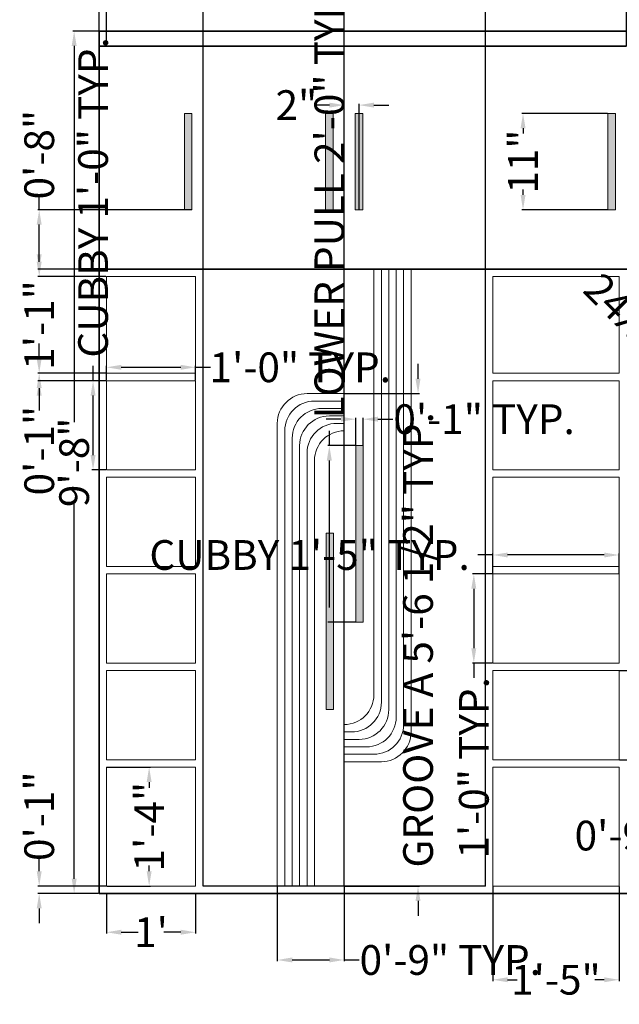
# Model space of a CAD drawing. Units: inches. Extents: x 13 to 156, y 156 to 357.
# Tile 1 of 3: x 13 to 94, y 156 to 289. Entities that reach past the tile are written whole.
import ezdxf

# ---------------------------------------------------------------- set-up
doc = ezdxf.new("R2010")
doc.units = ezdxf.units.IN
doc.header["$MEASUREMENT"] = 0
for name, color, linetype, lineweight in [('A-ANNO-DIMS', 2, 'Continuous', 18), ('A-FURN-CASE', 7, 'Continuous', 35), ('A-FURN-GRVE', 8, 'Continuous', 13), ('A-FURN-HDWR', 9, 'Continuous', 18), ('A-FURN-PANL', 7, 'Continuous', 25), ('A-FURN-SHLF', 7, 'Continuous', 18)]:
    doc.layers.add(name, color=color, linetype=linetype, lineweight=lineweight)
doc.styles.get("Standard").update_dxf_attribs({"font": 'arial.ttf'})
doc.dimstyles.get("Standard").update_dxf_attribs({"dimtxt": 4, "dimasz": 2, "dimexe": 0.18, "dimexo": 0.0625, "dimgap": 0.09, "dimtad": 0, "dimdec": 0, "dimzin": 0, "dimdsep": 46, "dimlunit": 4, "dimtxsty": 'Standard', "dimcen": 0.09, "dimadec": 0, "dimazin": 0, "dimtfac": 1, "dimtdec": 0, "dimtofl": 0, "dimtmove": 0, "dimatfit": 3, "dimfxl": 1, "dimtolj": 1, "dimtzin": 0, "dimarcsym": 0})

# ---------------------------------------------------------------- blocks, each defined once
blk = doc.blocks.new('*D1')
at = {"layer": 'A-ANNO-DIMS', "color": 0, "lineweight": -2, "transparency": 16777216}
for p, q in [((23.63, 285.13), (23.63, 305.65)), ((25.63, 305.47), (73.22, 305.47)), ((131.63, 305.47), (84.03, 305.47)), ((133.63, 285.13), (133.63, 305.65))]:
    blk.add_line(p, q, dxfattribs=at)
at = {"layer": 'A-ANNO-DIMS', "color": 0, "transparency": 16777216}
for points in [[(25.63, 305.81), (25.63, 305.14), (23.63, 305.47)], [(131.63, 305.81), (131.63, 305.14), (133.63, 305.47)]]:
    blk.add_solid(points, dxfattribs=at)
at = {"layer": 'Defpoints', "color": 0, "transparency": 16777216}
for p in [(133.63, 305.47), (23.63, 285.07), (133.63, 285.07)]:
    blk.add_point(p, dxfattribs=at)
at = {"layer": 'A-ANNO-DIMS', "color": 0, "transparency": 16777216, "insert": (78.63, 305.47), "char_height": 4, "attachment_point": 5}
blk.add_mtext('\\A1;9\'-2"', dxfattribs=at)
blk = doc.blocks.new('*D2')
at = {"layer": 'A-ANNO-DIMS', "color": 0, "lineweight": -2, "transparency": 16777216}
for p, q in [((21.63, 312.2), (19.63, 312.2)), ((23.63, 285.13), (23.63, 312.38)), ((24.63, 285.13), (24.63, 312.38)), ((26.63, 312.2), (28.63, 312.2))]:
    blk.add_line(p, q, dxfattribs=at)
at = {"layer": 'A-ANNO-DIMS', "color": 0, "transparency": 16777216}
for points in [[(21.63, 312.54), (21.63, 311.87), (23.63, 312.2)], [(26.63, 312.54), (26.63, 311.87), (24.63, 312.2)]]:
    blk.add_solid(points, dxfattribs=at)
at = {"layer": 'Defpoints', "color": 0, "transparency": 16777216}
for p in [(24.63, 312.2), (23.63, 285.07), (24.63, 285.07)]:
    blk.add_point(p, dxfattribs=at)
at = {"layer": 'A-ANNO-DIMS', "color": 0, "transparency": 16777216, "insert": (30.83, 312.2), "char_height": 4, "attachment_point": 5}
blk.add_mtext('\\A1;1"', dxfattribs=at)
blk = doc.blocks.new('*D3')
at = {"layer": 'A-ANNO-DIMS', "color": 0, "lineweight": -2, "transparency": 16777216}
for p, q in [((24.63, 171.01), (24.63, 165.68)), ((36.63, 171.01), (36.63, 165.68)), ((26.63, 165.86), (28.88, 165.86)), ((34.63, 165.86), (32.37, 165.86))]:
    blk.add_line(p, q, dxfattribs=at)
at = {"layer": 'A-ANNO-DIMS', "color": 0, "transparency": 16777216}
for points in [[(26.63, 166.2), (26.63, 165.53), (24.63, 165.86)], [(34.63, 166.2), (34.63, 165.53), (36.63, 165.86)]]:
    blk.add_solid(points, dxfattribs=at)
at = {"layer": 'Defpoints', "color": 0, "transparency": 16777216}
for p in [(24.63, 171.07), (36.63, 171.07), (36.63, 165.86)]:
    blk.add_point(p, dxfattribs=at)
at = {"layer": 'A-ANNO-DIMS', "color": 0, "transparency": 16777216, "insert": (30.63, 165.86), "char_height": 4, "attachment_point": 5}
blk.add_mtext("\\A1;1'", dxfattribs=at)
blk = doc.blocks.new('FDGHJKL')
h = blk.add_hatch(color=256)
h.dxf.hatch_style = 1
h.paths.add_polyline_path([(167.31, 269.36), (166.3, 269.36), (166.3, 256.4), (167.31, 256.4)])
blk.add_lwpolyline([(166.3, 269.36), (167.31, 269.36), (167.31, 256.4), (166.3, 256.4)], close=True)
blk = doc.blocks.new('CVBNM')
h = blk.add_hatch(color=256)
h.dxf.hatch_style = 1
h.paths.add_polyline_path([(77.18, 559), (76.19, 559), (76.19, 535.24), (77.18, 535.24)])
blk.add_lwpolyline([(76.19, 559), (76.19, 535.24), (77.18, 535.24), (77.18, 559)], close=True)
blk = doc.blocks.new('*D6')
at = {"layer": 'A-ANNO-DIMS', "color": 0, "lineweight": -2, "transparency": 16777216}
for p, q in [((54.63, 277.15), (52.63, 277.15)), ((56.63, 255.13), (56.63, 277.33)), ((58.63, 263.13), (58.63, 277.33)), ((60.63, 277.15), (62.63, 277.15))]:
    blk.add_line(p, q, dxfattribs=at)
at = {"layer": 'A-ANNO-DIMS', "color": 0, "transparency": 16777216}
for points in [[(54.63, 277.48), (54.63, 276.81), (56.63, 277.15)], [(60.63, 277.48), (60.63, 276.81), (58.63, 277.15)]]:
    blk.add_solid(points, dxfattribs=at)
at = {"layer": 'Defpoints', "color": 0, "transparency": 16777216}
for p in [(56.63, 277.15), (58.63, 263.07), (56.63, 255.07)]:
    blk.add_point(p, dxfattribs=at)
at = {"layer": 'A-ANNO-DIMS', "color": 0, "transparency": 16777216, "insert": (50.2, 277.15), "char_height": 4, "attachment_point": 5}
blk.add_mtext('\\A1;2"', dxfattribs=at)
blk = doc.blocks.new('*D7')
at = {"layer": 'A-ANNO-DIMS', "color": 0, "lineweight": -2, "transparency": 16777216}
for p, q in [((24.69, 188.07), (30.56, 188.07)), ((30.38, 186.07), (30.38, 185.29)), ((30.38, 174.07), (30.38, 174.85)), ((24.69, 172.07), (30.56, 172.07))]:
    blk.add_line(p, q, dxfattribs=at)
at = {"layer": 'A-ANNO-DIMS', "color": 0, "transparency": 16777216}
for points in [[(30.04, 186.07), (30.71, 186.07), (30.38, 188.07)], [(30.04, 174.07), (30.71, 174.07), (30.38, 172.07)]]:
    blk.add_solid(points, dxfattribs=at)
at = {"layer": 'Defpoints', "color": 0, "transparency": 16777216}
for p in [(24.63, 188.07), (30.38, 188.07), (24.63, 172.07)]:
    blk.add_point(p, dxfattribs=at)
at = {"layer": 'A-ANNO-DIMS', "color": 0, "transparency": 16777216, "insert": (30.38, 180.07), "char_height": 4, "attachment_point": 5, "rotation": 90}
blk.add_mtext('\\A1;1\'-4"', dxfattribs=at)
blk = doc.blocks.new('*D8')
at = {"layer": 'A-ANNO-DIMS', "color": 0, "lineweight": -2, "transparency": 16777216}
for p, q in [((76.63, 172.01), (76.63, 159.29)), ((93.63, 172.01), (93.63, 159.29)), ((78.63, 159.47), (79.91, 159.47)), ((91.63, 159.47), (90.35, 159.47))]:
    blk.add_line(p, q, dxfattribs=at)
at = {"layer": 'A-ANNO-DIMS', "color": 0, "transparency": 16777216}
for points in [[(78.63, 159.8), (78.63, 159.14), (76.63, 159.47)], [(91.63, 159.8), (91.63, 159.14), (93.63, 159.47)]]:
    blk.add_solid(points, dxfattribs=at)
at = {"layer": 'Defpoints', "color": 0, "transparency": 16777216}
for p in [(76.63, 172.07), (93.63, 172.07), (76.63, 159.47)]:
    blk.add_point(p, dxfattribs=at)
at = {"layer": 'A-ANNO-DIMS', "color": 0, "transparency": 16777216, "insert": (85.13, 159.47), "char_height": 4, "attachment_point": 5}
blk.add_mtext('\\A1;1\'-5"', dxfattribs=at)
blk = doc.blocks.new('*D9')
at = {"layer": 'A-ANNO-DIMS', "color": 0, "lineweight": -2, "transparency": 16777216}
for p, q in [((93.69, 201.07), (98.38, 201.07)), ((98.2, 199.07), (98.2, 196.81)), ((98.2, 191.07), (98.2, 193.33)), ((93.69, 189.07), (98.38, 189.07))]:
    blk.add_line(p, q, dxfattribs=at)
at = {"layer": 'A-ANNO-DIMS', "color": 0, "transparency": 16777216}
for points in [[(97.87, 199.07), (98.53, 199.07), (98.2, 201.07)], [(97.87, 191.07), (98.53, 191.07), (98.2, 189.07)]]:
    blk.add_solid(points, dxfattribs=at)
at = {"layer": 'Defpoints', "color": 0, "transparency": 16777216}
for p in [(93.63, 201.07), (98.2, 201.07), (93.63, 189.07)]:
    blk.add_point(p, dxfattribs=at)
at = {"layer": 'A-ANNO-DIMS', "color": 0, "transparency": 16777216, "insert": (98.2, 195.07), "char_height": 4, "attachment_point": 5, "rotation": 90}
blk.add_mtext("\\A1;1'", dxfattribs=at)
blk = doc.blocks.new('*D11')
at = {"layer": 'A-ANNO-DIMS', "color": 0, "lineweight": -2, "transparency": 16777216}
for p, q in [((92.06, 276.03), (80.52, 276.03)), ((80.7, 274.03), (80.7, 273.31)), ((80.7, 265.07), (80.7, 265.8)), ((92.06, 263.07), (80.52, 263.07))]:
    blk.add_line(p, q, dxfattribs=at)
at = {"layer": 'A-ANNO-DIMS', "color": 0, "transparency": 16777216}
for points in [[(80.37, 274.03), (81.04, 274.03), (80.7, 276.03)], [(80.37, 265.07), (81.04, 265.07), (80.7, 263.07)]]:
    blk.add_solid(points, dxfattribs=at)
at = {"layer": 'Defpoints', "color": 0, "transparency": 16777216}
for p in [(80.7, 276.03), (92.12, 276.03), (92.12, 263.07)]:
    blk.add_point(p, dxfattribs=at)
at = {"layer": 'A-ANNO-DIMS', "color": 0, "transparency": 16777216, "insert": (80.7, 269.55), "char_height": 4, "attachment_point": 5, "rotation": 90}
blk.add_mtext('\\A1;11"', dxfattribs=at)
blk = doc.blocks.new('*D12')
at = {"layer": 'A-ANNO-DIMS', "color": 0, "lineweight": -2, "transparency": 16777216}
for p, q in [((23.56, 287.11), (20.1, 287.11)), ((20.28, 285.11), (20.28, 234.5)), ((20.28, 173.07), (20.28, 223.68)), ((23.56, 171.07), (20.1, 171.07))]:
    blk.add_line(p, q, dxfattribs=at)
at = {"layer": 'A-ANNO-DIMS', "color": 0, "transparency": 16777216}
for points in [[(19.95, 285.11), (20.62, 285.11), (20.28, 287.11)], [(19.95, 173.07), (20.62, 173.07), (20.28, 171.07)]]:
    blk.add_solid(points, dxfattribs=at)
at = {"layer": 'Defpoints', "color": 0, "transparency": 16777216}
for p in [(23.63, 287.11), (20.28, 171.07), (23.63, 171.07)]:
    blk.add_point(p, dxfattribs=at)
at = {"layer": 'A-ANNO-DIMS', "color": 0, "transparency": 16777216, "insert": (20.28, 229.09), "char_height": 4, "attachment_point": 5, "rotation": 90}
blk.add_mtext('\\A1;9\'-8"', dxfattribs=at)
blk = doc.blocks.new('WDR-CUBBY-12X12')
for p, q in [((12, 12), (0, 12)), ((0, 0), (0, 12)), ((12, 0), (12, 12)), ((12, 0), (0, 0))]:
    blk.add_line(p, q)
blk = doc.blocks.new('WDR-CUBBY-17X12')
for p, q in [((17, 12), (0, 12)), ((0, 0), (0, 12)), ((17, 0), (17, 12)), ((17, 0), (0, 0))]:
    blk.add_line(p, q)
blk = doc.blocks.new('WDR-GROOVE-PANEL-A')
for p, q in [((9, 66.26), (4, 66.26)), ((9, 65.26), (5, 65.26)), ((9, 64.26), (6, 64.26)), ((9, 63.26), (7, 63.26)), ((0, 62.26), (0, 0)), ((1, 61.26), (1, 0)), ((9, 62.26), (8, 62.26)), ((9, 61.26), (9, 61.26)), ((2, 60.26), (2, 0)), ((3, 59.26), (3, 0)), ((4, 58.26), (4, 0)), ((5, 57.26), (5, 0))]:
    blk.add_line(p, q)
for centre in [(4, 62.26), (5, 61.26), (6, 60.26), (7, 59.26), (8, 58.26), (9, 57.26)]:
    blk.add_arc(centre, 4, 90, 180)
blk = doc.blocks.new('*D21')
at = {"layer": 'A-ANNO-DIMS', "color": 0, "lineweight": -2, "transparency": 16777216}
for p, q in [((54.63, 231.33), (54.63, 233.33)), ((58.13, 231.33), (54.45, 231.33)), ((54.63, 209.57), (54.63, 229.33)), ((58.13, 207.57), (54.45, 207.57))]:
    blk.add_line(p, q, dxfattribs=at)
at = {"layer": 'A-ANNO-DIMS', "color": 0, "transparency": 16777216}
for points in [[(54.29, 229.33), (54.96, 229.33), (54.63, 231.33)], [(54.29, 209.57), (54.96, 209.57), (54.63, 207.57)]]:
    blk.add_solid(points, dxfattribs=at)
at = {"layer": 'Defpoints', "color": 0, "transparency": 16777216}
for p in [(54.63, 231.33), (58.19, 231.33), (58.19, 207.57)]:
    blk.add_point(p, dxfattribs=at)
at = {"layer": 'A-ANNO-DIMS', "color": 0, "transparency": 16777216, "insert": (54.63, 264.31), "char_height": 4, "attachment_point": 5, "rotation": 90}
blk.add_mtext('\\A1;LOWER PULL 2\'-0" TYP.', dxfattribs=at)
blk = doc.blocks.new('*D22')
at = {"layer": 'A-ANNO-DIMS', "color": 0, "lineweight": -2, "transparency": 16777216}
for p, q in [((56.19, 234.89), (54.19, 234.89)), ((58.19, 231.39), (58.19, 235.07)), ((59.18, 231.39), (59.18, 235.07)), ((61.18, 234.89), (63.18, 234.89))]:
    blk.add_line(p, q, dxfattribs=at)
at = {"layer": 'A-ANNO-DIMS', "color": 0, "transparency": 16777216}
for points in [[(56.19, 235.23), (56.19, 234.56), (58.19, 234.89)], [(61.18, 235.23), (61.18, 234.56), (59.18, 234.89)]]:
    blk.add_solid(points, dxfattribs=at)
at = {"layer": 'Defpoints', "color": 0, "transparency": 16777216}
for p in [(59.18, 234.89), (58.19, 231.33), (59.18, 231.33)]:
    blk.add_point(p, dxfattribs=at)
at = {"layer": 'A-ANNO-DIMS', "color": 0, "transparency": 16777216, "insert": (75.46, 234.89), "char_height": 4, "attachment_point": 5}
blk.add_mtext('\\A1;0\'-1" TYP.', dxfattribs=at)
blk = doc.blocks.new('*D23')
at = {"layer": 'A-ANNO-DIMS', "color": 0, "lineweight": -2, "transparency": 16777216}
for p, q in [((66.57, 240.33), (66.57, 242.33)), ((56.69, 238.33), (66.75, 238.33)), ((56.69, 172.07), (66.75, 172.07)), ((66.57, 170.07), (66.57, 168.07))]:
    blk.add_line(p, q, dxfattribs=at)
at = {"layer": 'A-ANNO-DIMS', "color": 0, "transparency": 16777216}
for points in [[(66.23, 240.33), (66.9, 240.33), (66.57, 238.33)], [(66.23, 170.07), (66.9, 170.07), (66.57, 172.07)]]:
    blk.add_solid(points, dxfattribs=at)
at = {"layer": 'Defpoints', "color": 0, "transparency": 16777216}
for p in [(56.63, 238.33), (66.57, 238.33), (56.63, 172.07)]:
    blk.add_point(p, dxfattribs=at)
at = {"layer": 'A-ANNO-DIMS', "color": 0, "transparency": 16777216, "insert": (66.57, 205.2), "char_height": 4, "attachment_point": 5, "rotation": 90}
blk.add_mtext('\\A1;GROOVE A 5\'-6 1/2" TYP.', dxfattribs=at)
blk = doc.blocks.new('*D24')
at = {"layer": 'A-ANNO-DIMS', "color": 0, "lineweight": -2, "transparency": 16777216}
for p, q in [((47.63, 172.01), (47.63, 161.95)), ((56.63, 172.01), (56.63, 161.95)), ((49.63, 162.13), (54.63, 162.13)), ((56.63, 162.13), (58.63, 162.13))]:
    blk.add_line(p, q, dxfattribs=at)
at = {"layer": 'A-ANNO-DIMS', "color": 0, "transparency": 16777216}
for points in [[(49.63, 162.47), (49.63, 161.8), (47.63, 162.13)], [(54.63, 162.47), (54.63, 161.8), (56.63, 162.13)]]:
    blk.add_solid(points, dxfattribs=at)
at = {"layer": 'Defpoints', "color": 0, "transparency": 16777216}
for p in [(47.63, 172.07), (56.63, 172.07), (56.63, 162.13)]:
    blk.add_point(p, dxfattribs=at)
at = {"layer": 'A-ANNO-DIMS', "color": 0, "transparency": 16777216, "insert": (70.91, 162.13), "char_height": 4, "attachment_point": 5}
blk.add_mtext('\\A1;0\'-9" TYP.', dxfattribs=at)
blk = doc.blocks.new('*D26')
at = {"layer": 'A-ANNO-DIMS', "color": 0, "lineweight": -2, "transparency": 16777216}
for p, q in [((114.13, 188.75), (114.13, 178.69)), ((123.13, 188.75), (123.13, 178.69)), ((114.13, 178.87), (112.13, 178.87)), ((121.13, 178.87), (116.13, 178.87))]:
    blk.add_line(p, q, dxfattribs=at)
at = {"layer": 'A-ANNO-DIMS', "color": 0, "transparency": 16777216}
for points in [[(116.13, 179.21), (116.13, 178.54), (114.13, 178.87)], [(121.13, 179.21), (121.13, 178.54), (123.13, 178.87)]]:
    blk.add_solid(points, dxfattribs=at)
at = {"layer": 'Defpoints', "color": 0, "transparency": 16777216}
for p in [(114.13, 188.81), (123.13, 188.81), (114.13, 178.87)]:
    blk.add_point(p, dxfattribs=at)
at = {"layer": 'A-ANNO-DIMS', "color": 0, "transparency": 16777216, "insert": (99.85, 178.87), "char_height": 4, "attachment_point": 5}
blk.add_mtext('\\A1;0\'-9" TYP.', dxfattribs=at)
blk = doc.blocks.new('*D27')
at = {"layer": 'A-ANNO-DIMS', "color": 0, "lineweight": -2, "transparency": 16777216}
for p, q in [((22.83, 240.07), (22.83, 242.07)), ((24.56, 240.07), (22.65, 240.07)), ((22.83, 230.07), (22.83, 238.07)), ((24.56, 228.07), (22.65, 228.07))]:
    blk.add_line(p, q, dxfattribs=at)
at = {"layer": 'A-ANNO-DIMS', "color": 0, "transparency": 16777216}
for points in [[(22.49, 238.07), (23.16, 238.07), (22.83, 240.07)], [(22.49, 230.07), (23.16, 230.07), (22.83, 228.07)]]:
    blk.add_solid(points, dxfattribs=at)
at = {"layer": 'Defpoints', "color": 0, "transparency": 16777216}
for p in [(22.83, 240.07), (24.63, 240.07), (24.63, 228.07)]:
    blk.add_point(p, dxfattribs=at)
at = {"layer": 'A-ANNO-DIMS', "color": 0, "transparency": 16777216, "insert": (22.83, 264.73), "char_height": 4, "attachment_point": 5, "rotation": 90}
blk.add_mtext('\\A1;CUBBY 1\'-0" TYP.', dxfattribs=at)
blk = doc.blocks.new('*D28')
at = {"layer": 'A-ANNO-DIMS', "color": 0, "lineweight": -2, "transparency": 16777216}
for p, q in [((24.63, 240.13), (24.63, 242.05)), ((26.63, 241.87), (34.63, 241.87)), ((36.63, 240.13), (36.63, 242.05)), ((36.63, 241.87), (38.63, 241.87))]:
    blk.add_line(p, q, dxfattribs=at)
at = {"layer": 'A-ANNO-DIMS', "color": 0, "transparency": 16777216}
for points in [[(26.63, 242.2), (26.63, 241.54), (24.63, 241.87)], [(34.63, 242.2), (34.63, 241.54), (36.63, 241.87)]]:
    blk.add_solid(points, dxfattribs=at)
at = {"layer": 'Defpoints', "color": 0, "transparency": 16777216}
for p in [(36.63, 241.87), (24.63, 240.07), (36.63, 240.07)]:
    blk.add_point(p, dxfattribs=at)
at = {"layer": 'A-ANNO-DIMS', "color": 0, "transparency": 16777216, "insert": (50.72, 241.87), "char_height": 4, "attachment_point": 5}
blk.add_mtext('\\A1;1\'-0" TYP.', dxfattribs=at)
blk = doc.blocks.new('*D29')
at = {"layer": 'A-ANNO-DIMS', "color": 0, "lineweight": -2, "transparency": 16777216}
for p, q in [((76.63, 216.62), (74.63, 216.62)), ((76.63, 214.13), (76.63, 216.8)), ((91.63, 216.62), (78.63, 216.62)), ((93.63, 214.13), (93.63, 216.8))]:
    blk.add_line(p, q, dxfattribs=at)
at = {"layer": 'A-ANNO-DIMS', "color": 0, "transparency": 16777216}
for points in [[(78.63, 216.95), (78.63, 216.29), (76.63, 216.62)], [(91.63, 216.95), (91.63, 216.29), (93.63, 216.62)]]:
    blk.add_solid(points, dxfattribs=at)
at = {"layer": 'Defpoints', "color": 0, "transparency": 16777216}
for p in [(76.63, 216.62), (76.63, 214.07), (93.63, 214.07)]:
    blk.add_point(p, dxfattribs=at)
at = {"layer": 'A-ANNO-DIMS', "color": 0, "transparency": 16777216, "insert": (51.97, 216.62), "char_height": 4, "attachment_point": 5}
blk.add_mtext('\\A1;CUBBY 1\'-5" TYP.', dxfattribs=at)
blk = doc.blocks.new('*D30')
at = {"layer": 'A-ANNO-DIMS', "color": 0, "lineweight": -2, "transparency": 16777216}
for p, q in [((76.56, 214.07), (73.9, 214.07)), ((74.08, 212.07), (74.08, 204.07)), ((76.56, 202.07), (73.9, 202.07)), ((74.08, 202.07), (74.08, 200.07))]:
    blk.add_line(p, q, dxfattribs=at)
at = {"layer": 'A-ANNO-DIMS', "color": 0, "transparency": 16777216}
for points in [[(73.74, 212.07), (74.41, 212.07), (74.08, 214.07)], [(73.74, 204.07), (74.41, 204.07), (74.08, 202.07)]]:
    blk.add_solid(points, dxfattribs=at)
at = {"layer": 'Defpoints', "color": 0, "transparency": 16777216}
for p in [(76.63, 214.07), (74.08, 202.07), (76.63, 202.07)]:
    blk.add_point(p, dxfattribs=at)
at = {"layer": 'A-ANNO-DIMS', "color": 0, "transparency": 16777216, "insert": (74.08, 187.98), "char_height": 4, "attachment_point": 5, "rotation": 90}
blk.add_mtext('\\A1;1\'-0" TYP.', dxfattribs=at)
blk = doc.blocks.new('*D31')
at = {"layer": 'A-ANNO-DIMS', "color": 0, "lineweight": -2, "transparency": 16777216}
for p, q in [((21.63, 295.16), (19.63, 295.16)), ((23.63, 285.13), (23.63, 295.34)), ((37.63, 285.13), (37.63, 295.34)), ((39.63, 295.16), (41.63, 295.16))]:
    blk.add_line(p, q, dxfattribs=at)
at = {"layer": 'A-ANNO-DIMS', "color": 0, "transparency": 16777216}
for points in [[(21.63, 295.49), (21.63, 294.82), (23.63, 295.16)], [(39.63, 295.49), (39.63, 294.82), (37.63, 295.16)]]:
    blk.add_solid(points, dxfattribs=at)
at = {"layer": 'Defpoints', "color": 0, "transparency": 16777216}
for p in [(37.63, 295.16), (23.63, 285.07), (37.63, 285.07)]:
    blk.add_point(p, dxfattribs=at)
at = {"layer": 'A-ANNO-DIMS', "color": 0, "transparency": 16777216, "insert": (30.63, 295.16), "char_height": 4, "attachment_point": 5}
blk.add_mtext('\\A1;1\'-2"', dxfattribs=at)
blk = doc.blocks.new('*D32')
at = {"layer": 'A-ANNO-DIMS', "color": 0, "lineweight": -2, "transparency": 16777216}
for p, q in [((37.63, 285.13), (37.63, 295.34)), ((39.63, 295.16), (41.91, 295.16)), ((54.63, 295.16), (52.35, 295.16)), ((56.63, 285.13), (56.63, 295.34))]:
    blk.add_line(p, q, dxfattribs=at)
at = {"layer": 'A-ANNO-DIMS', "color": 0, "transparency": 16777216}
for points in [[(39.63, 295.49), (39.63, 294.82), (37.63, 295.16)], [(54.63, 295.49), (54.63, 294.82), (56.63, 295.16)]]:
    blk.add_solid(points, dxfattribs=at)
at = {"layer": 'Defpoints', "color": 0, "transparency": 16777216}
for p in [(56.63, 295.16), (37.63, 285.07), (56.63, 285.07)]:
    blk.add_point(p, dxfattribs=at)
at = {"layer": 'A-ANNO-DIMS', "color": 0, "transparency": 16777216, "insert": (47.13, 295.16), "char_height": 4, "attachment_point": 5}
blk.add_mtext('\\A1;1\'-7"', dxfattribs=at)
blk = doc.blocks.new('*D33')
at = {"layer": 'A-ANNO-DIMS', "color": 0, "lineweight": -2, "transparency": 16777216}
for p, q in [((56.63, 285.13), (56.63, 295.34)), ((58.63, 295.16), (60.91, 295.16)), ((73.63, 295.16), (71.35, 295.16)), ((75.63, 285.13), (75.63, 295.34))]:
    blk.add_line(p, q, dxfattribs=at)
at = {"layer": 'A-ANNO-DIMS', "color": 0, "transparency": 16777216}
for points in [[(58.63, 295.49), (58.63, 294.82), (56.63, 295.16)], [(73.63, 295.49), (73.63, 294.82), (75.63, 295.16)]]:
    blk.add_solid(points, dxfattribs=at)
at = {"layer": 'Defpoints', "color": 0, "transparency": 16777216}
for p in [(75.63, 295.16), (56.63, 285.07), (75.63, 285.07)]:
    blk.add_point(p, dxfattribs=at)
at = {"layer": 'A-ANNO-DIMS', "color": 0, "transparency": 16777216, "insert": (66.13, 295.16), "char_height": 4, "attachment_point": 5}
blk.add_mtext('\\A1;1\'-7"', dxfattribs=at)
blk = doc.blocks.new('*D34')
at = {"layer": 'A-ANNO-DIMS', "color": 0, "lineweight": -2, "transparency": 16777216}
for p, q in [((75.63, 285.13), (75.63, 295.34)), ((77.63, 295.16), (79.91, 295.16)), ((92.63, 295.16), (90.35, 295.16)), ((94.63, 285.13), (94.63, 295.34))]:
    blk.add_line(p, q, dxfattribs=at)
at = {"layer": 'A-ANNO-DIMS', "color": 0, "transparency": 16777216}
for points in [[(77.63, 295.49), (77.63, 294.82), (75.63, 295.16)], [(92.63, 295.49), (92.63, 294.82), (94.63, 295.16)]]:
    blk.add_solid(points, dxfattribs=at)
at = {"layer": 'Defpoints', "color": 0, "transparency": 16777216}
for p in [(94.63, 295.16), (75.63, 285.07), (94.63, 285.07)]:
    blk.add_point(p, dxfattribs=at)
at = {"layer": 'A-ANNO-DIMS', "color": 0, "transparency": 16777216, "insert": (85.13, 295.16), "char_height": 4, "attachment_point": 5}
blk.add_mtext('\\A1;1\'-7"', dxfattribs=at)
blk = doc.blocks.new('*D38')
at = {"layer": 'A-ANNO-DIMS', "color": 0, "lineweight": -2, "transparency": 16777216}
for p, q in [((15.58, 174.07), (15.58, 176.07)), ((24.56, 172.07), (15.4, 172.07)), ((23.56, 171.07), (15.4, 171.07)), ((15.58, 169.07), (15.58, 167.07))]:
    blk.add_line(p, q, dxfattribs=at)
at = {"layer": 'A-ANNO-DIMS', "color": 0, "transparency": 16777216}
for points in [[(15.24, 174.07), (15.91, 174.07), (15.58, 172.07)], [(15.24, 169.07), (15.91, 169.07), (15.58, 171.07)]]:
    blk.add_solid(points, dxfattribs=at)
at = {"layer": 'Defpoints', "color": 0, "transparency": 16777216}
for p in [(15.58, 172.07), (23.63, 171.07), (24.63, 172.07)]:
    blk.add_point(p, dxfattribs=at)
at = {"layer": 'A-ANNO-DIMS', "color": 0, "transparency": 16777216, "insert": (15.58, 181.48), "char_height": 4, "attachment_point": 5, "rotation": 90}
blk.add_mtext('\\A1;0\'-1"', dxfattribs=at)
blk = doc.blocks.new('*D39')
at = {"layer": 'A-ANNO-DIMS', "color": 0, "lineweight": -2, "transparency": 16777216}
for p, q in [((15.58, 256.07), (15.58, 258.07)), ((24.56, 254.07), (15.4, 254.07)), ((24.56, 241.07), (15.4, 241.07)), ((15.58, 239.07), (15.58, 237.07))]:
    blk.add_line(p, q, dxfattribs=at)
at = {"layer": 'A-ANNO-DIMS', "color": 0, "transparency": 16777216}
for points in [[(15.24, 256.07), (15.91, 256.07), (15.58, 254.07)], [(15.24, 239.07), (15.91, 239.07), (15.58, 241.07)]]:
    blk.add_solid(points, dxfattribs=at)
at = {"layer": 'Defpoints', "color": 0, "transparency": 16777216}
for p in [(24.63, 254.07), (15.58, 241.07), (24.63, 241.07)]:
    blk.add_point(p, dxfattribs=at)
at = {"layer": 'A-ANNO-DIMS', "color": 0, "transparency": 16777216, "insert": (15.58, 247.57), "char_height": 4, "attachment_point": 5, "rotation": 90}
blk.add_mtext('\\A1;1\'-1"', dxfattribs=at)
blk = doc.blocks.new('*D40')
at = {"layer": 'A-ANNO-DIMS', "color": 0, "lineweight": -2, "transparency": 16777216}
for p, q in [((15.58, 243.07), (15.58, 245.07)), ((24.56, 241.07), (15.4, 241.07)), ((24.56, 240.07), (15.4, 240.07)), ((15.58, 238.07), (15.58, 236.07))]:
    blk.add_line(p, q, dxfattribs=at)
at = {"layer": 'A-ANNO-DIMS', "color": 0, "transparency": 16777216}
for points in [[(15.24, 243.07), (15.91, 243.07), (15.58, 241.07)], [(15.24, 238.07), (15.91, 238.07), (15.58, 240.07)]]:
    blk.add_solid(points, dxfattribs=at)
at = {"layer": 'Defpoints', "color": 0, "transparency": 16777216}
for p in [(15.58, 240.07), (24.63, 241.07), (24.63, 240.07)]:
    blk.add_point(p, dxfattribs=at)
at = {"layer": 'A-ANNO-DIMS', "color": 0, "transparency": 16777216, "insert": (15.58, 230.66), "char_height": 4, "attachment_point": 5, "rotation": 90}
blk.add_mtext('\\A1;0\'-1"', dxfattribs=at)
blk = doc.blocks.new('*D41')
at = {"layer": 'A-ANNO-DIMS', "color": 0, "lineweight": -2, "transparency": 16777216}
for p, q in [((15.58, 263.07), (15.58, 265.07)), ((36.07, 263.07), (15.4, 263.07)), ((15.58, 257.07), (15.58, 261.07)), ((37.56, 255.07), (15.4, 255.07))]:
    blk.add_line(p, q, dxfattribs=at)
at = {"layer": 'A-ANNO-DIMS', "color": 0, "transparency": 16777216}
for points in [[(15.24, 261.07), (15.91, 261.07), (15.58, 263.07)], [(15.24, 257.07), (15.91, 257.07), (15.58, 255.07)]]:
    blk.add_solid(points, dxfattribs=at)
at = {"layer": 'Defpoints', "color": 0, "transparency": 16777216}
for p in [(15.58, 263.07), (36.13, 263.07), (37.63, 255.07)]:
    blk.add_point(p, dxfattribs=at)
at = {"layer": 'A-ANNO-DIMS', "color": 0, "transparency": 16777216, "insert": (15.58, 270.48), "char_height": 4, "attachment_point": 5, "rotation": 90}
blk.add_mtext('\\A1;0\'-8"', dxfattribs=at)
blk = doc.blocks.new('*D45')
at = {"layer": 'A-ANNO-DIMS', "color": 0, "lineweight": -2, "transparency": 16777216}
for p, q in [((108.47, 234.99), (109.89, 233.58)), ((114.04, 229.33), (114.22, 229.33)), ((114.13, 229.24), (114.13, 229.42))]:
    blk.add_line(p, q, dxfattribs=at)
at = {"layer": 'A-ANNO-DIMS', "color": 0, "transparency": 16777216}
blk.add_solid([(110.12, 233.81), (109.65, 233.34), (111.3, 232.16)], dxfattribs=at)
at = {"layer": 'Defpoints', "color": 0, "transparency": 16777216}
for p in [(111.3, 232.16), (114.13, 229.33)]:
    blk.add_point(p, dxfattribs=at)
at = {"layer": 'A-ANNO-DIMS', "color": 0, "transparency": 16777216, "insert": (99.14, 244.33), "char_height": 4, "attachment_point": 5, "rotation": 314.9766}
blk.add_mtext('\\A1;24X R0\'-4"', dxfattribs=at)

msp = doc.modelspace()

# ---------------------------------------------------------------- linework, layer by layer
at = {"layer": 'A-FURN-CASE'}
for p, q in [((23.63, 171.07), (23.63, 287.11)), ((23.63, 287.11), (94.63, 287.11)), ((23.63, 285.07), (94.63, 285.07)), ((23.63, 255.07), (133.63, 255.07)), ((133.63, 171.07), (23.63, 171.07))]:
    msp.add_line(p, q, dxfattribs=at)
at = {"layer": 'A-FURN-PANL'}
for p, q in [((37.63, 255.07), (37.63, 285.07)), ((56.63, 255.07), (56.63, 285.07)), ((75.63, 255.07), (75.63, 285.07)), ((37.63, 172.07), (37.63, 255.07)), ((56.63, 172.07), (56.63, 255.07)), ((75.63, 172.07), (75.63, 255.07)), ((75.63, 172.07), (37.63, 172.07))]:
    msp.add_line(p, q, dxfattribs=at)
at = {"layer": 'A-FURN-SHLF'}
for p, q in [((24.63, 241.07), (24.63, 254.07)), ((24.63, 254.07), (36.63, 254.07)), ((36.63, 241.07), (36.63, 254.07)), ((76.63, 241.07), (76.63, 254.07)), ((76.63, 254.07), (93.63, 254.07)), ((93.63, 241.07), (93.63, 254.07)), ((36.63, 241.07), (24.63, 241.07)), ((93.63, 241.07), (76.63, 241.07)), ((24.63, 172.07), (24.63, 188.07)), ((36.63, 188.07), (24.63, 188.07)), ((36.63, 172.07), (36.63, 188.07)), ((76.63, 172.07), (76.63, 188.07)), ((93.63, 188.07), (76.63, 188.07)), ((93.63, 172.07), (93.63, 188.07)), ((36.63, 172.07), (24.63, 172.07)), ((93.63, 172.07), (76.63, 172.07))]:
    msp.add_line(p, q, dxfattribs=at)

# ---------------------------------------------------------------- block references
at = {"layer": 'A-FURN-GRVE', "rotation": 180}
msp.add_blockref('WDR-GROOVE-PANEL-A', (65.63, 255.07), dxfattribs=at)
at = {"layer": 'A-FURN-GRVE'}
msp.add_blockref('WDR-GROOVE-PANEL-A', (47.63, 172.07), dxfattribs=at)
at = {"layer": 'A-FURN-HDWR'}
for name, p in [('FDGHJKL', (-131.18, 6.67)), ('FDGHJKL', (-112.18, 6.67)), ('FDGHJKL', (-108.18, 6.67)), ('FDGHJKL', (-74.18, 6.67)), ('CVBNM', (-18, -327.67)), ('CVBNM', (-22, -339.43))]:
    msp.add_blockref(name, p, dxfattribs=at)
at = {"layer": 'A-FURN-SHLF'}
for name, p in [('WDR-CUBBY-12X12', (24.63, 228.07)), ('WDR-CUBBY-17X12', (76.63, 228.07))]:
    msp.add_blockref(name, p, dxfattribs=at)
for name, p, rotation in [('WDR-CUBBY-12X12', (36.63, 215.07), 90.00000000000003), ('WDR-CUBBY-17X12', (93.63, 227.07), 180), ('WDR-CUBBY-12X12', (36.63, 202.07), 90.0000000000001), ('WDR-CUBBY-17X12', (93.63, 214.07), 180), ('WDR-CUBBY-12X12', (36.63, 189.07), 90.00000000000048), ('WDR-CUBBY-17X12', (93.63, 201.07), 180)]:
    msp.add_blockref(name, p, dxfattribs=dict(at, rotation=rotation))

# ---------------------------------------------------------------- dimensions: what is measured, and where the dimension line sits
at = {"layer": 'A-ANNO-DIMS'}
for base, p1, p2, override, picture, middle in [((24.63, 312.2), (23.63, 285.07), (24.63, 285.07), {"dimclrd": 0, "dimclre": 0, "dimclrt": 0}, '*D2', (30.83, 312.2)), ((133.63, 305.47), (23.63, 285.07), (133.63, 285.07), {"dimclrd": 0, "dimclre": 0, "dimclrt": 0}, '*D1', (78.63, 305.47)), ((37.63, 295.16), (23.63, 285.07), (37.63, 285.07), {"dimdec": 1, "dimlfac": 1, "dimrnd": 0, "dimzin": 1, "dimdsep": 46, "dimlunit": 4, "dimfrac": 2}, '*D31', (30.63, 295.16)), ((56.63, 295.16), (37.63, 285.07), (56.63, 285.07), {"dimdec": 1, "dimlfac": 1, "dimrnd": 0, "dimzin": 1, "dimdsep": 46, "dimlunit": 4, "dimfrac": 2}, '*D32', (47.13, 295.16)), ((75.63, 295.16), (56.63, 285.07), (75.63, 285.07), {"dimdec": 1, "dimlfac": 1, "dimrnd": 0, "dimzin": 1, "dimdsep": 46, "dimlunit": 4, "dimfrac": 2}, '*D33', (66.13, 295.16)), ((94.63, 295.16), (75.63, 285.07), (94.63, 285.07), {"dimdec": 1, "dimlfac": 1, "dimrnd": 0, "dimzin": 1, "dimdsep": 46, "dimlunit": 4, "dimfrac": 2}, '*D34', (85.13, 295.16)), ((56.63, 277.15), (58.63, 263.07), (56.63, 255.07), {"dimclrd": 0, "dimclre": 0, "dimclrt": 0}, '*D6', (50.2, 277.15)), ((36.63, 165.86), (24.63, 171.07), (36.63, 171.07), {"dimclrd": 0, "dimclre": 0, "dimclrt": 0}, '*D3', (30.63, 165.86)), ((76.63, 159.47), (93.63, 172.07), (76.63, 172.07), {"dimclrd": 0, "dimclre": 0, "dimclrt": 0}, '*D8', (85.13, 159.47))]:
    dim = msp.add_linear_dim(base=base, p1=p1, p2=p2, dimstyle='Standard', override=override, dxfattribs=at)
    dim.commit()
    dim.dimension.update_dxf_attribs({"geometry": picture, "text_midpoint": middle})
for base, p1, p2, angle, text, override, picture, middle in [((54.63, 231.33), (58.19, 207.57), (58.19, 231.33), 90, 'LOWER PULL <> TYP.', {"dimdec": 1, "dimlfac": 1, "dimrnd": 0, "dimzin": 1, "dimdsep": 46, "dimlunit": 4, "dimfrac": 2}, '*D21', (54.63, 264.31)), ((22.83, 240.07), (24.63, 228.07), (24.63, 240.07), 90, 'CUBBY <> TYP.', {"dimdec": 1, "dimlfac": 1, "dimrnd": 0, "dimzin": 1, "dimdsep": 46, "dimlunit": 4, "dimfrac": 2}, '*D27', (22.83, 264.73)), ((80.7, 276.03), (92.12, 263.07), (92.12, 276.03), 90, '11"', {"dimclrd": 0, "dimclre": 0, "dimclrt": 0}, '*D11', (80.7, 269.55)), ((66.57, 238.33), (56.63, 172.07), (56.63, 238.33), 90, 'GROOVE A <> TYP.', {"dimdec": 1, "dimlfac": 1, "dimrnd": 0, "dimzin": 1, "dimdsep": 46, "dimlunit": 4, "dimfrac": 2}, '*D23', (66.57, 205.2)), ((76.63, 216.62), (93.63, 214.07), (76.63, 214.07), 180, 'CUBBY <> TYP.', {"dimdec": 1, "dimlfac": 1, "dimrnd": 0, "dimzin": 1, "dimdsep": 46, "dimlunit": 4, "dimfrac": 2}, '*D29', (51.97, 216.62)), ((74.08, 202.07), (76.63, 214.07), (76.63, 202.07), 270, '<> TYP.', {"dimdec": 1, "dimlfac": 1, "dimrnd": 0, "dimzin": 1, "dimdsep": 46, "dimlunit": 4, "dimfrac": 2}, '*D30', (74.08, 187.98)), ((114.13, 178.87), (123.13, 188.81), (114.13, 188.81), 180, '<> TYP.', {"dimdec": 1, "dimlfac": 1, "dimrnd": 0, "dimzin": 1, "dimdsep": 46, "dimlunit": 4, "dimfrac": 2}, '*D26', (99.85, 178.87))]:
    dim = msp.add_linear_dim(base=base, p1=p1, p2=p2, angle=angle, text=text, dimstyle='Standard', override=override, dxfattribs=at)
    dim.commit()
    dim.dimension.update_dxf_attribs({"geometry": picture, "text_midpoint": middle})
for base, p1, p2, override, picture, middle in [((20.28, 171.07), (23.63, 287.11), (23.63, 171.07), {"dimclrd": 0, "dimclre": 0, "dimclrt": 0}, '*D12', (20.28, 229.09)), ((15.58, 263.07), (37.63, 255.07), (36.13, 263.07), {"dimdec": 1, "dimlfac": 1, "dimrnd": 0, "dimzin": 1, "dimdsep": 46, "dimlunit": 4, "dimfrac": 2}, '*D41', (15.58, 270.48)), ((15.58, 241.07), (24.63, 254.07), (24.63, 241.07), {"dimdec": 1, "dimlfac": 1, "dimrnd": 0, "dimzin": 1, "dimdsep": 46, "dimlunit": 4, "dimfrac": 2}, '*D39', (15.58, 247.57)), ((15.58, 240.07), (24.63, 241.07), (24.63, 240.07), {"dimdec": 1, "dimlfac": 1, "dimrnd": 0, "dimzin": 1, "dimdsep": 46, "dimlunit": 4, "dimfrac": 2}, '*D40', (15.58, 230.66)), ((98.2, 201.07), (93.63, 189.07), (93.63, 201.07), {"dimclrd": 0, "dimclre": 0, "dimclrt": 0}, '*D9', (98.2, 195.07)), ((15.58, 172.07), (23.63, 171.07), (24.63, 172.07), {"dimdec": 1, "dimlfac": 1, "dimrnd": 0, "dimzin": 1, "dimdsep": 46, "dimlunit": 4, "dimfrac": 2}, '*D38', (15.58, 181.48)), ((30.38, 188.07), (24.63, 172.07), (24.63, 188.07), {"dimclrd": 0, "dimclre": 0, "dimclrt": 0}, '*D7', (30.38, 180.07))]:
    dim = msp.add_linear_dim(base=base, p1=p1, p2=p2, angle=90, dimstyle='Standard', override=override, dxfattribs=at)
    dim.commit()
    dim.dimension.update_dxf_attribs({"geometry": picture, "text_midpoint": middle})
dim = msp.add_radius_dim(center=(114.13, 229.33), mpoint=(111.3, 232.16), text='24X <>', dimstyle='Standard', override={"dimdec": 1, "dimlfac": 1, "dimrnd": 0, "dimzin": 1, "dimdsep": 46, "dimlunit": 4, "dimfrac": 2}, dxfattribs=at)
dim.commit()
dim.dimension.update_dxf_attribs({"geometry": '*D45', "text_midpoint": (99.14, 244.33)})
for base, p1, p2, picture, middle in [((36.63, 241.87), (24.63, 240.07), (36.63, 240.07), '*D28', (50.72, 241.87)), ((59.18, 234.89), (58.19, 231.33), (59.18, 231.33), '*D22', (75.46, 234.89)), ((56.63, 162.13), (47.63, 172.07), (56.63, 172.07), '*D24', (70.91, 162.13))]:
    dim = msp.add_linear_dim(base=base, p1=p1, p2=p2, text='<> TYP.', dimstyle='Standard', override={"dimdec": 1, "dimlfac": 1, "dimrnd": 0, "dimzin": 1, "dimdsep": 46, "dimlunit": 4, "dimfrac": 2}, dxfattribs=at)
    dim.commit()
    dim.dimension.update_dxf_attribs({"geometry": picture, "text_midpoint": middle})

doc.saveas('drawing.dxf')
